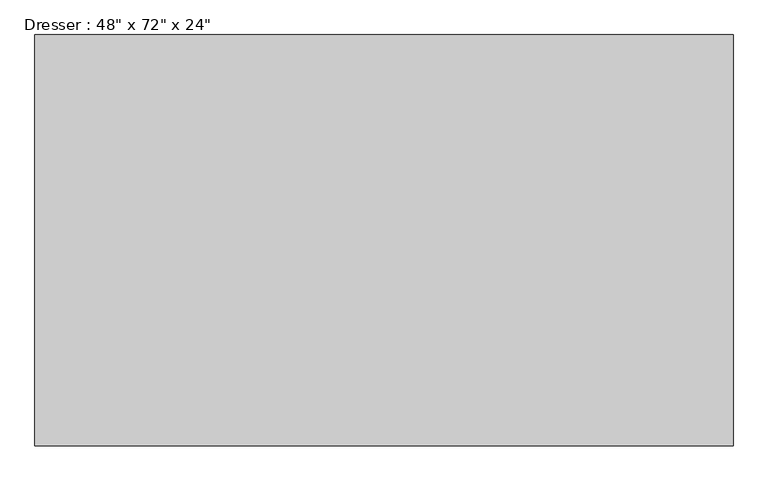
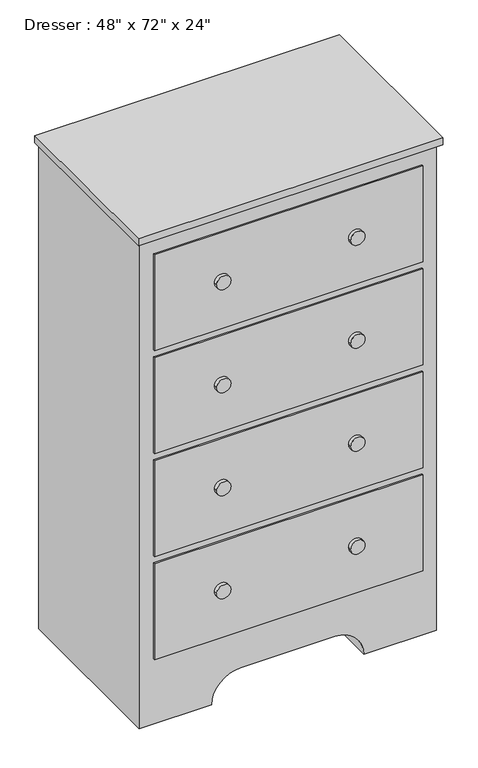
"""IFC4 building model written with IfcOpenShell, lengths in millimetres: furniture geometry."""

from ifc_helpers import new_model, si_unit, point, frame, frame_2d, origin, place, context, project, spatial, polyline, circle_curve, trimmed, segment, composite_curve, outline, extrude, source, transform, mapped, element, save


def furniture_f72bdee3(model_context):
    return source(origin(), model_context, "Body", "SweptSolid", [
        extrude(outline(polyline([(264.2067402, -58.3629541), (264.2067402, -687.0129541), (-802.5932598, -687.0129541), (-802.5932598, -58.3629541), (264.2067402, -58.3629541)])), frame((0.0, 0.0, 1803.4), z_axis=(0.0, 0.0, 1.0), x_axis=(1.0, 0.0, 0.0)), (0.0, 0.0, 1.0), 25.4),
        extrude(outline(composite_curve([segment(polyline([(0.0, 251.5067402), (1803.4, 251.5067402), (1803.4, -789.8932598), (0.0, -789.8932598), (0.0, -535.8932598)]), True, "CONTINUOUS"), segment(trimmed(circle_curve(frame_2d((0.0, -434.2932598)), 101.6), [point((0.0, -535.8932598))], [point((101.6, -434.2932598))], True, "CARTESIAN"), True, "CONTINUOUS"), segment(polyline([(101.6, -434.2932598), (101.6, -104.0932598)]), True, "CONTINUOUS"), segment(trimmed(circle_curve(frame_2d((0.0, -104.0932598)), 101.6), [point((101.6, -104.0932598))], [point((0.0, -2.4932598))], True, "CARTESIAN"), True, "CONTINUOUS"), segment(polyline([(0.0, -2.4932598), (0.0, 251.5067402)]), True, "CONTINUOUS")], self_intersect=False)), frame((0.0, -667.9629541, 0.0), z_axis=(0.0, 1.0, 0.0), x_axis=(0.0, 0.0, 1.0)), (0.0, 0.0, 1.0), 609.6),
        extrude(outline(composite_curve([segment(trimmed(circle_curve(frame_2d((1562.1, -34.2432598)), 25.4), [point((1562.1, -59.6432598))], [point((1562.1, -8.8432598))], False, "CARTESIAN"), True, "CONTINUOUS"), segment(trimmed(circle_curve(frame_2d((1562.1, -34.2432598)), 25.4), [point((1562.1, -8.8432598))], [point((1562.1, -59.6432598))], False, "CARTESIAN"), True, "CONTINUOUS")], self_intersect=False)), frame((0.0, -687.0129541, 0.0), z_axis=(0.0, 1.0, 0.0), x_axis=(0.0, 0.0, 1.0)), (0.0, 0.0, 1.0), 12.7),
        extrude(outline(composite_curve([segment(trimmed(circle_curve(frame_2d((1181.1, -34.2432598)), 25.4), [point((1181.1, -59.6432598))], [point((1181.1, -8.8432598))], False, "CARTESIAN"), True, "CONTINUOUS"), segment(trimmed(circle_curve(frame_2d((1181.1, -34.2432598)), 25.4), [point((1181.1, -8.8432598))], [point((1181.1, -59.6432598))], False, "CARTESIAN"), True, "CONTINUOUS")], self_intersect=False)), frame((0.0, -687.0129541, 0.0), z_axis=(0.0, 1.0, 0.0), x_axis=(0.0, 0.0, 1.0)), (0.0, 0.0, 1.0), 12.7),
        extrude(outline(composite_curve([segment(trimmed(circle_curve(frame_2d((800.1, -34.2432598)), 25.4), [point((800.1, -59.6432598))], [point((800.1, -8.8432598))], False, "CARTESIAN"), True, "CONTINUOUS"), segment(trimmed(circle_curve(frame_2d((800.1, -34.2432598)), 25.4), [point((800.1, -8.8432598))], [point((800.1, -59.6432598))], False, "CARTESIAN"), True, "CONTINUOUS")], self_intersect=False)), frame((0.0, -687.0129541, 0.0), z_axis=(0.0, 1.0, 0.0), x_axis=(0.0, 0.0, 1.0)), (0.0, 0.0, 1.0), 12.7),
        extrude(outline(composite_curve([segment(trimmed(circle_curve(frame_2d((419.1, -34.2432598)), 25.4), [point((419.1, -59.6432598))], [point((419.1, -8.8432598))], False, "CARTESIAN"), True, "CONTINUOUS"), segment(trimmed(circle_curve(frame_2d((419.1, -34.2432598)), 25.4), [point((419.1, -8.8432598))], [point((419.1, -59.6432598))], False, "CARTESIAN"), True, "CONTINUOUS")], self_intersect=False)), frame((0.0, -687.0129541, 0.0), z_axis=(0.0, 1.0, 0.0), x_axis=(0.0, 0.0, 1.0)), (0.0, 0.0, 1.0), 12.7),
        extrude(outline(composite_curve([segment(trimmed(circle_curve(frame_2d((419.1, -504.1432598)), 25.4), [point((419.1, -529.5432598))], [point((419.1, -478.7432598))], False, "CARTESIAN"), True, "CONTINUOUS"), segment(trimmed(circle_curve(frame_2d((419.1, -504.1432598)), 25.4), [point((419.1, -478.7432598))], [point((419.1, -529.5432598))], False, "CARTESIAN"), True, "CONTINUOUS")], self_intersect=False)), frame((0.0, -687.0129541, 0.0), z_axis=(0.0, 1.0, 0.0), x_axis=(0.0, 0.0, 1.0)), (0.0, 0.0, 1.0), 12.7),
        extrude(outline(composite_curve([segment(trimmed(circle_curve(frame_2d((800.1, -504.1432598)), 25.4), [point((800.1, -529.5432598))], [point((800.1, -478.7432598))], False, "CARTESIAN"), True, "CONTINUOUS"), segment(trimmed(circle_curve(frame_2d((800.1, -504.1432598)), 25.4), [point((800.1, -478.7432598))], [point((800.1, -529.5432598))], False, "CARTESIAN"), True, "CONTINUOUS")], self_intersect=False)), frame((0.0, -687.0129541, 0.0), z_axis=(0.0, 1.0, 0.0), x_axis=(0.0, 0.0, 1.0)), (0.0, 0.0, 1.0), 12.7),
        extrude(outline(composite_curve([segment(trimmed(circle_curve(frame_2d((1181.1, -504.1432598)), 25.4), [point((1181.1, -529.5432598))], [point((1181.1, -478.7432598))], False, "CARTESIAN"), True, "CONTINUOUS"), segment(trimmed(circle_curve(frame_2d((1181.1, -504.1432598)), 25.4), [point((1181.1, -478.7432598))], [point((1181.1, -529.5432598))], False, "CARTESIAN"), True, "CONTINUOUS")], self_intersect=False)), frame((0.0, -687.0129541, 0.0), z_axis=(0.0, 1.0, 0.0), x_axis=(0.0, 0.0, 1.0)), (0.0, 0.0, 1.0), 12.7),
        extrude(outline(composite_curve([segment(trimmed(circle_curve(frame_2d((1562.1, -504.1432598)), 25.4), [point((1562.1, -529.5432598))], [point((1562.1, -478.7432598))], False, "CARTESIAN"), True, "CONTINUOUS"), segment(trimmed(circle_curve(frame_2d((1562.1, -504.1432598)), 25.4), [point((1562.1, -478.7432598))], [point((1562.1, -529.5432598))], False, "CARTESIAN"), True, "CONTINUOUS")], self_intersect=False)), frame((0.0, -687.0129541, 0.0), z_axis=(0.0, 1.0, 0.0), x_axis=(0.0, 0.0, 1.0)), (0.0, 0.0, 1.0), 12.7),
        extrude(outline(polyline([(200.7067402, -674.3129541), (-739.0932598, -674.3129541), (-739.0932598, -667.9629541), (200.7067402, -667.9629541), (200.7067402, -674.3129541)])), frame((0.0, 0.0, 1384.3), z_axis=(0.0, 0.0, 1.0), x_axis=(1.0, 0.0, 0.0)), (0.0, 0.0, 1.0), 355.6),
        extrude(outline(polyline([(200.7067402, -674.3129541), (-739.0932598, -674.3129541), (-739.0932598, -667.9629541), (200.7067402, -667.9629541), (200.7067402, -674.3129541)])), frame((0.0, 0.0, 1003.3), z_axis=(0.0, 0.0, 1.0), x_axis=(1.0, 0.0, 0.0)), (0.0, 0.0, 1.0), 355.6),
        extrude(outline(polyline([(200.7067402, -674.3129541), (-739.0932598, -674.3129541), (-739.0932598, -667.9629541), (200.7067402, -667.9629541), (200.7067402, -674.3129541)])), frame((0.0, 0.0, 622.3), z_axis=(0.0, 0.0, 1.0), x_axis=(1.0, 0.0, 0.0)), (0.0, 0.0, 1.0), 355.6),
        extrude(outline(polyline([(200.7067402, -674.3129541), (-739.0932598, -674.3129541), (-739.0932598, -667.9629541), (200.7067402, -667.9629541), (200.7067402, -674.3129541)])), frame((0.0, 0.0, 241.3), z_axis=(0.0, 0.0, 1.0), x_axis=(1.0, 0.0, 0.0)), (0.0, 0.0, 1.0), 355.6),
    ])


if __name__ == "__main__":
    model = new_model("IFC4")
    model_context = context("Model", 3, world=origin())
    ifc_project = project(units=[si_unit("LENGTHUNIT", "METRE", prefix="MILLI")], contexts=[model_context])
    site = spatial("IfcSite", under=ifc_project)
    building = spatial("IfcBuilding", under=site)
    placement = place(None, origin())
    furniture_shape = furniture_f72bdee3(model_context)
    element("IfcFurniture", 1, ObjectType="Dresser : 48\" x 72\" x 24\"", at=placement, inside=building, context=model_context, shape_type="MappedRepresentation", body=[
        mapped(furniture_shape, transform((0.0, 0.0, 0.0), x_axis=(1.0, 0.0, 0.0), y_axis=(0.0, 1.0, 0.0), z_axis=(0.0, 0.0, 1.0))),
    ])
    save(model, "model.ifc")

# Revit data of these elements
# Type "Dresser : 48\" x 72\" x 24\""
#   Assembly Code = "E2020200"
#   Depth = 2' - 0"
#   Height = 6' - 0"
#   Width = 3' - 5"
#   Dresser Material = Laminate - Ivory, Glossy
#   Drawer Material = Laminate, Ivory, Matte
#   Knob Material = Cherry
#   Default Elevation = 0
# Element 1 (IfcFurniture, "Dresser : 48\" x 72\" x 24\"")
#   Materials on its faces: "Laminate, Ivory, Matte", "Cherry", "Laminate - Ivory, Glossy"
# Materials
#   "Laminate - Ivory, Glossy": colour RGB 247 247 239, transparency 0
#   "Laminate, Ivory, Matte": class "Plastic", colour RGB 247 247 239, transparency 0, Description = "Plastic Laminate - Ivory, Matte", Cost = 0
#   "Cherry": class "Wood", colour RGB 226 177 128, transparency 0, Description = "Prunus Serotina", Cost = 0
